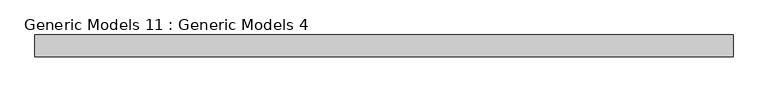
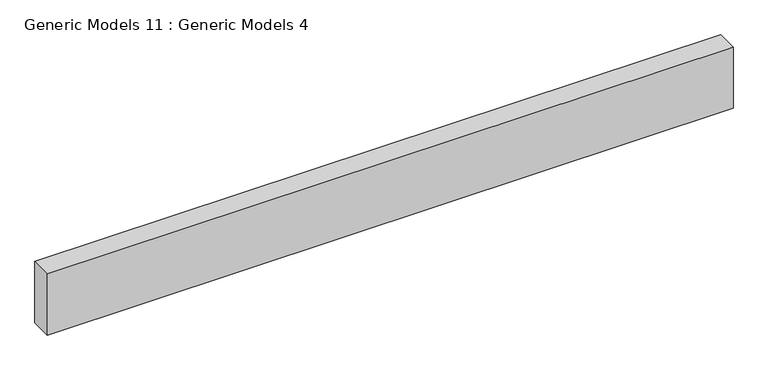
"""IFC4 building model written with IfcOpenShell, lengths in millimetres: proxy geometry, Generic Models 11 : Generic Models 4."""

from ifc_helpers import new_model, si_unit, frame, origin, place, context, project, spatial, polyline, outline, extrude, source, transform, mapped, element, save


def generic_models_11_generic_models_4_fdae65e2(model_context):
    return source(origin(), model_context, "Body", "SweptSolid", [
        extrude(outline(polyline([(-5569.5456086, -11268.8679047), (-10418.2707824, -11268.8679047), (-10418.2707824, -11116.4679047), (-5569.5456086, -11116.4679047), (-5569.5456086, -11268.8679047)])), frame((0.0, 0.0, 12039.6), z_axis=(0.0, 0.0, 1.0), x_axis=(1.0, 0.0, 0.0)), (0.0, 0.0, 1.0), 457.2),
    ])


if __name__ == "__main__":
    model = new_model("IFC4")
    model_context = context("Model", 3, world=origin())
    ifc_project = project(units=[si_unit("LENGTHUNIT", "METRE", prefix="MILLI")], contexts=[model_context])
    site = spatial("IfcSite", under=ifc_project)
    building = spatial("IfcBuilding", under=site)
    placement = place(None, origin())
    generic_models_11_generic_models_4_shape = generic_models_11_generic_models_4_fdae65e2(model_context)
    element("IfcBuildingElementProxy", 1, Name="Generic Models 11 : Generic Models 4", ObjectType="Generic Models 11 : Generic Models 4", at=placement, inside=building, context=model_context, shape_type="MappedRepresentation", body=[
        mapped(generic_models_11_generic_models_4_shape, transform((0.0, 0.0, 0.0), x_axis=(1.0, 0.0, 0.0), y_axis=(0.0, 1.0, 0.0), z_axis=(0.0, 0.0, 1.0))),
    ])
    save(model, "model.ifc")

# Revit data of these elements
# Element 1 (IfcBuildingElementProxy, "Generic Models 11 : Generic Models 4")
#   Materials on its faces: "WALL ACCENT 6\""
# Materials
#   "WALL ACCENT 6\"": class "Generic", colour RGB 120 120 120, transparency 0, Cost = 0
